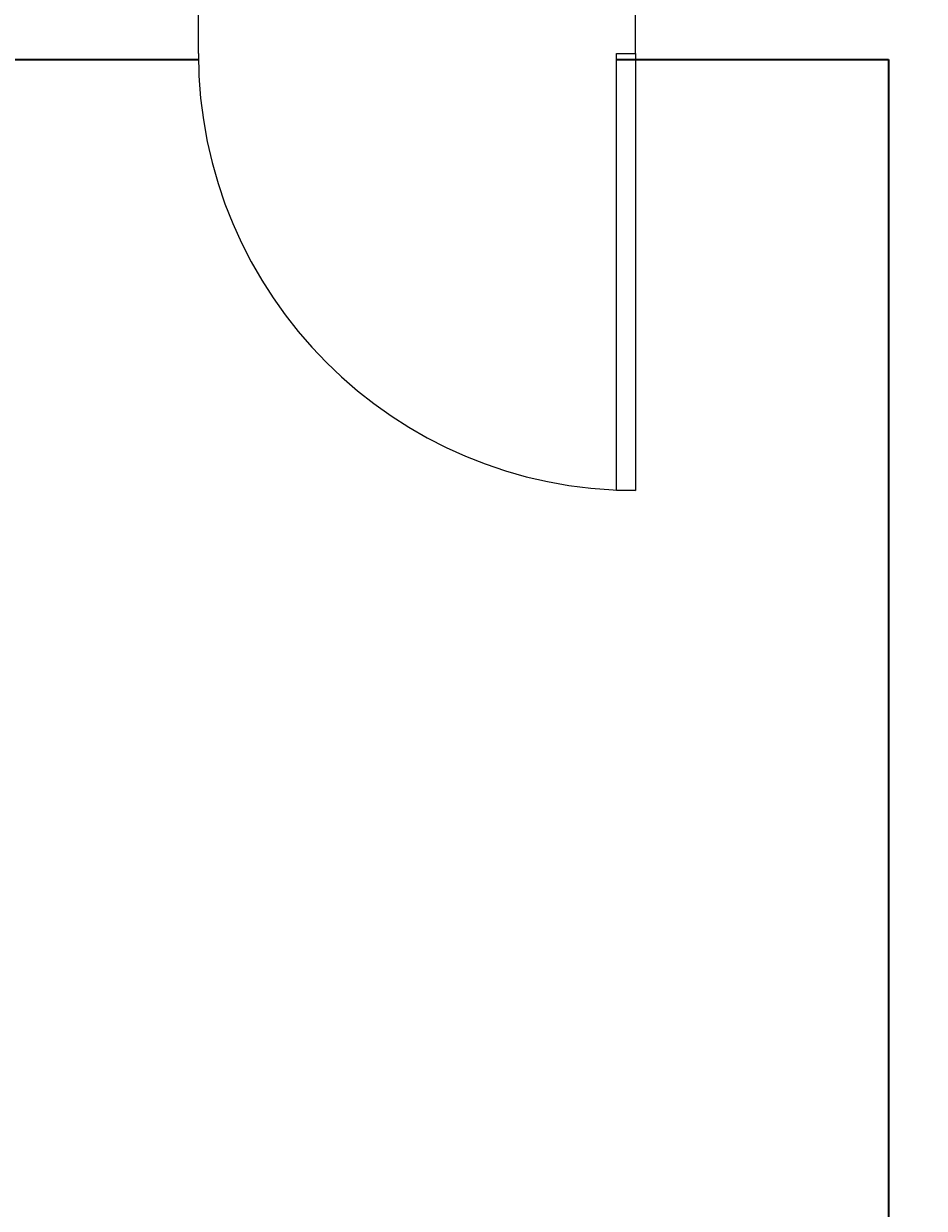
# Model space of a CAD drawing. Units: millimetres. Extents: x 27017497 to 27018854, y 7058029 to 7059154.
# Tile 29 of 91: x 27017748 to 27017804, y 7058222 to 7058297. Entities that reach past the tile are written whole.
import ezdxf

# ---------------------------------------------------------------- set-up
doc = ezdxf.new("R2010")
doc.units = ezdxf.units.MM
for name, color, linetype, lineweight in [('A-ANNO-DIMS', 2, 'Continuous', 18), ('A-DOOR', 4, 'Continuous', 20), ('A-WALL', 7, 'Continuous', 35)]:
    doc.layers.add(name, color=color, linetype=linetype, lineweight=lineweight)
doc.styles.get("Standard").update_dxf_attribs({"font": 'arial.ttf'})
doc.dimstyles.get("Standard").update_dxf_attribs({"dimtxt": 0.18, "dimasz": 0.18, "dimexe": 0.18, "dimexo": 0.0625, "dimgap": 0.09, "dimtad": 0, "dimtih": 1, "dimtoh": 1, "dimdec": 4, "dimzin": 0, "dimdsep": 46, "dimtxsty": 'Standard', "dimcen": 0.09, "dimadec": 0, "dimazin": 0, "dimtfac": 1, "dimtdec": 4, "dimtofl": 0, "dimtmove": 0, "dimatfit": 3, "dimfxl": 1, "dimtolj": 1, "dimtzin": 0, "dimarcsym": 0})

# ---------------------------------------------------------------- blocks, each defined once
blk = doc.blocks.new('*U2')
for p, q in [((0, 0), (0, -6)), ((40, 0), (40, -6))]:
    blk.add_line(p, q)
blk.add_lwpolyline([(0, 0), (0, 40), (1.75, 40), (1.75, 0)], close=True)
blk.add_arc((0, 0), 40, 0, 90)
blk = doc.blocks.new('*D47')
at = {"layer": 'A-ANNO-DIMS', "color": 0, "lineweight": -2, "transparency": 16777216}
for p, q in [((27017561.166, 7058294.35), (27017561.166, 7058028.6)), ((27018790.606, 7058294.35), (27018790.606, 7058028.6)), ((27017561.346, 7058028.78), (27018175.431, 7058028.78)), ((27018790.426, 7058028.78), (27018176.341, 7058028.78))]:
    blk.add_line(p, q, dxfattribs=at)
at = {"layer": 'A-ANNO-DIMS', "color": 0, "transparency": 16777216}
for points in [[(27017561.346, 7058028.81), (27017561.346, 7058028.75), (27017561.166, 7058028.78)], [(27018790.426, 7058028.81), (27018790.426, 7058028.75), (27018790.606, 7058028.78)]]:
    blk.add_solid(points, dxfattribs=at)
at = {"layer": 'Defpoints', "color": 0, "transparency": 16777216}
for p in [(27017561.166, 7058294.412), (27018790.606, 7058294.412), (27018790.606, 7058028.78)]:
    blk.add_point(p, dxfattribs=at)
at = {"layer": 'A-ANNO-DIMS', "color": 0, "transparency": 16777216, "insert": (27018175.886, 7058028.78), "char_height": 0.18, "attachment_point": 5}
blk.add_mtext('\\A1;1229.4', dxfattribs=at)
blk = doc.blocks.new('*D48')
at = {"layer": 'A-ANNO-DIMS', "color": 0, "lineweight": -2, "transparency": 16777216}
for p, q in [((27018463.498, 7058622.912), (27017497.536, 7058622.912)), ((27017497.716, 7058622.732), (27017497.716, 7058357.753)), ((27017497.716, 7058092.41), (27017497.716, 7058357.389)), ((27018555.129, 7058092.23), (27017497.536, 7058092.23))]:
    blk.add_line(p, q, dxfattribs=at)
at = {"layer": 'A-ANNO-DIMS', "color": 0, "transparency": 16777216}
for points in [[(27017497.686, 7058622.732), (27017497.746, 7058622.732), (27017497.716, 7058622.912)], [(27017497.686, 7058092.41), (27017497.746, 7058092.41), (27017497.716, 7058092.23)]]:
    blk.add_solid(points, dxfattribs=at)
at = {"layer": 'Defpoints', "color": 0, "transparency": 16777216}
for p in [(27018463.561, 7058622.912), (27017497.716, 7058092.23), (27018555.192, 7058092.23)]:
    blk.add_point(p, dxfattribs=at)
at = {"layer": 'A-ANNO-DIMS', "color": 0, "transparency": 16777216, "insert": (27017497.716, 7058357.571), "char_height": 0.18, "attachment_point": 5}
blk.add_mtext('\\A1;530.7', dxfattribs=at)

msp = doc.modelspace()

# ---------------------------------------------------------------- linework, layer by layer
at = {"layer": 'A-WALL'}
for p, q in [((27017622.666, 7058294.412), (27017758.765, 7058294.412)), ((27017785.044, 7058294.412), (27017802.166, 7058294.412)), ((27017802.166, 7058294.412), (27017802.166, 7058208.446))]:
    msp.add_line(p, q, dxfattribs=at)

# ---------------------------------------------------------------- block references
at = {"layer": 'A-DOOR', "xscale": 0.6870473523349573, "yscale": 0.6870473523349573, "zscale": 0.6870473523349573, "rotation": 180}
msp.add_blockref('*U2', (27017786.261, 7058294.793), dxfattribs=at)

# ---------------------------------------------------------------- dimensions: what is measured, and where the dimension line sits
at = {"layer": 'A-ANNO-DIMS'}
dim = msp.add_linear_dim(base=(27017497.716, 7058092.23), p1=(27018463.561, 7058622.912), p2=(27018555.192, 7058092.23), angle=90, dimstyle='Standard', override={"dimdec": 1, "dimlfac": 1, "dimrnd": 0, "dimzin": 0, "dimdsep": 46, "dimlunit": 2}, dxfattribs=at)
dim.commit()
dim.dimension.update_dxf_attribs({"geometry": '*D48', "text_midpoint": (27017497.716, 7058357.571)})
dim = msp.add_linear_dim(base=(27018790.606, 7058028.78), p1=(27017561.166, 7058294.412), p2=(27018790.606, 7058294.412), dimstyle='Standard', override={"dimdec": 1, "dimlfac": 1, "dimrnd": 0, "dimzin": 0, "dimdsep": 46, "dimlunit": 2}, dxfattribs=at)
dim.commit()
dim.dimension.update_dxf_attribs({"geometry": '*D47', "text_midpoint": (27018175.886, 7058028.78)})

doc.saveas('drawing.dxf')
